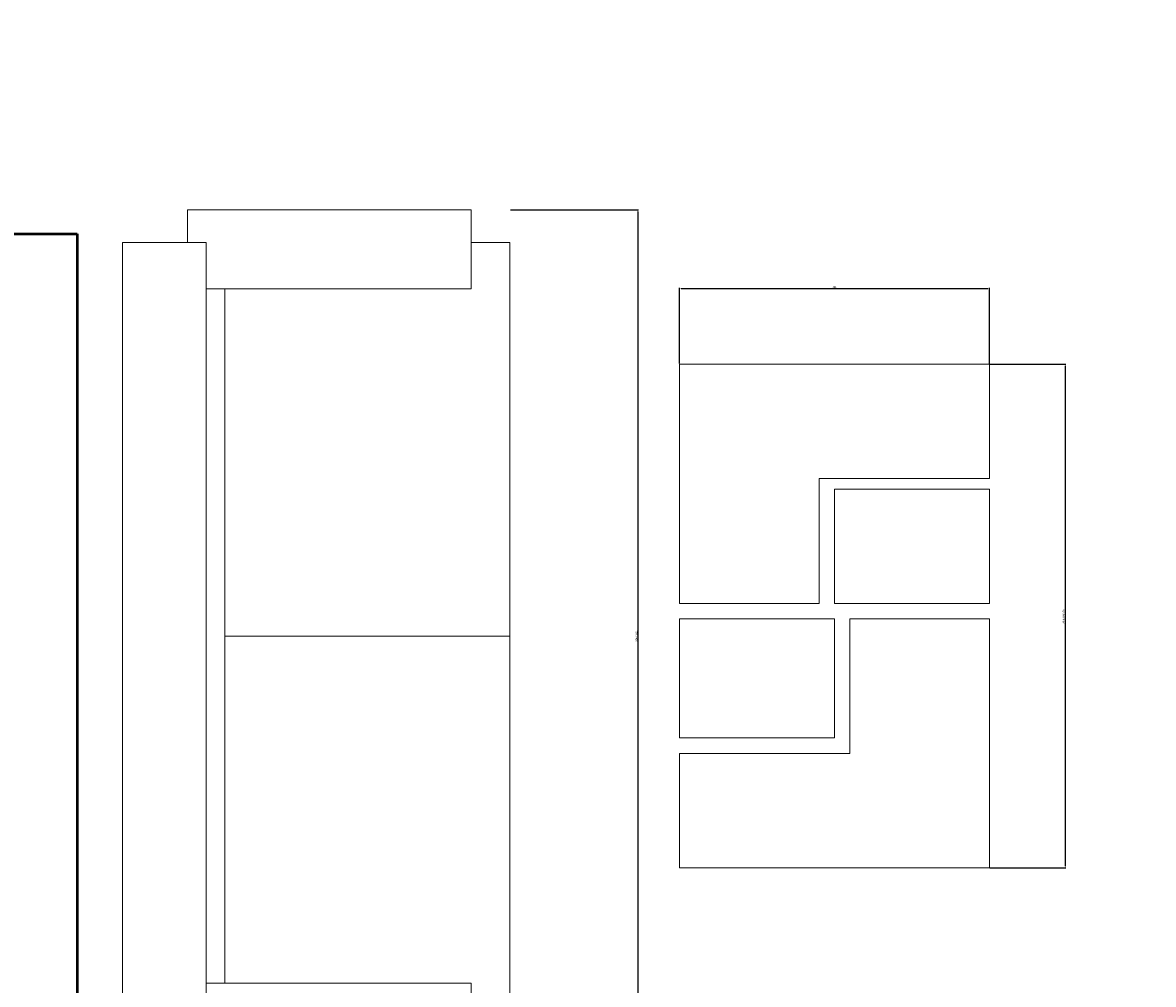
# Model space of a CAD drawing. Units: millimetres. Extents: x -857 to 54106, y -13666 to 13947.
# Tile 9 of 41: x 7333 to 9086, y 6990 to 8482. Entities that reach past the tile are written whole.
import ezdxf

# ---------------------------------------------------------------- set-up
doc = ezdxf.new("R2010")
doc.units = ezdxf.units.MM
for name, color, linetype, lineweight in [('A-ANNO-DIMS', 2, 'Continuous', 18), ('A-FLOR-PATT', 252, 'Continuous', 13), ('A-FURN', 21, 'Continuous', 18), ('A-FURNITURE', 25, 'Continuous', 9), ('A-WALL', 7, 'Continuous', 50)]:
    doc.layers.add(name, color=color, linetype=linetype, lineweight=lineweight)
doc.styles.get("Standard").update_dxf_attribs({"font": 'arial.ttf'})
doc.dimstyles.new('ISO-25', dxfattribs={"dimtxt": 2.5, "dimasz": 2.5, "dimexe": 1.25, "dimexo": 0.625, "dimtad": 1, "dimtxsty": 'Standard', "dimcen": 2.5, "dimadec": 0, "dimazin": 0, "dimtfac": 1, "dimtmove": 0, "dimatfit": 3, "dimfxl": 1, "dimarcsym": 0})

# ---------------------------------------------------------------- blocks, each defined once
blk = doc.blocks.new('A$C0E8E2537')
at = {"layer": 'A-FURNITURE'}
for p, q in [((30.478, 0), (-30.478, 0)), ((-30.478, 0), (-30.478, -6.486)), ((30.478, 0), (30.478, -6.486)), ((-30.478, -5.045), (-33, -5.045)), ((-33, -5.045), (-33, -26.997)), ((30.478, -5.045), (33, -5.045)), ((33, -5.045), (33, -26.997)), ((30.478, -6.486), (-30.478, -6.486)), ((-26.874, -6.486), (-26.874, -7.927)), ((26.874, -6.486), (26.874, -26.997)), ((26.874, -7.927), (-26.874, -7.927)), ((-26.874, -7.927), (-26.874, -26.997)), ((0, -30), (0, -7.927)), ((-33, -26.997), (-26.874, -26.997)), ((-30.478, -26.997), (-30.478, -30)), ((33, -26.997), (26.874, -26.997)), ((30.478, -26.997), (30.478, -30)), ((30.478, -30), (-30.478, -30))]:
    blk.add_line(p, q, dxfattribs=at)
blk = doc.blocks.new('A$C03AA15B9')
at = {"layer": 'A-FURNITURE'}
for points in [[(13.194, 19.718), (13.194, 30.14), (0, 30.14), (0, 38.992), (24, 38.992), (24, 19.718)], [(0, 28.945), (12, 28.945), (12, 19.718), (0, 19.718)], [(10.806, 18.524), (10.806, 8.852), (24, 8.852), (24, 0), (0, 0), (0, 18.524)], [(24, 9.672), (12, 9.672), (12, 18.524), (24, 18.524)]]:
    blk.add_lwpolyline(points, close=True, dxfattribs=at)
blk = doc.blocks.new('*D53')
at = {"layer": 'A-ANNO-DIMS', "color": 0, "lineweight": -2, "transparency": 16777216}
for p, q in [((8089.1, 8191.6), (8288, 8191.6)), ((8286.8, 8189.1), (8286.8, 6871.7)), ((8089.1, 6869.2), (8288, 6869.2))]:
    blk.add_line(p, q, dxfattribs=at)
at = {"layer": 'A-ANNO-DIMS', "color": 0, "transparency": 16777216}
for points in [[(8286.4, 8189.1), (8287.2, 8189.1), (8286.8, 8191.6)], [(8286.4, 6871.7), (8287.2, 6871.7), (8286.8, 6869.2)]]:
    blk.add_solid(points, dxfattribs=at)
at = {"layer": 'Defpoints', "color": 0, "transparency": 16777216}
for p in [(8088.4, 8191.6), (8088.4, 6869.2), (8286.8, 6869.2)]:
    blk.add_point(p, dxfattribs=at)
at = {"layer": 'A-ANNO-DIMS', "color": 0, "transparency": 16777216, "insert": (8284.9, 7530.4), "char_height": 2.5, "attachment_point": 5, "rotation": 90}
blk.add_mtext('SOFA 1322', dxfattribs=at)
blk = doc.blocks.new('*D55')
at = {"layer": 'A-ANNO-DIMS', "color": 0, "lineweight": -2, "transparency": 16777216}
for p, q in [((8832.8, 7952.3), (8950.6, 7952.3)), ((8949.3, 7949.8), (8949.3, 7173.6)), ((8832.8, 7171.1), (8950.6, 7171.1))]:
    blk.add_line(p, q, dxfattribs=at)
at = {"layer": 'A-ANNO-DIMS', "color": 0, "transparency": 16777216}
for points in [[(8948.9, 7949.8), (8949.8, 7949.8), (8949.3, 7952.3)], [(8948.9, 7173.6), (8949.8, 7173.6), (8949.3, 7171.1)]]:
    blk.add_solid(points, dxfattribs=at)
at = {"layer": 'Defpoints', "color": 0, "transparency": 16777216}
for p in [(8832.2, 7952.3), (8832.2, 7171.1), (8949.3, 7171.1)]:
    blk.add_point(p, dxfattribs=at)
at = {"layer": 'A-ANNO-DIMS', "color": 0, "transparency": 16777216, "insert": (8947.4, 7561.7), "char_height": 2.5, "attachment_point": 5, "rotation": 90}
blk.add_mtext('ARMCHAIR 781', dxfattribs=at)
blk = doc.blocks.new('*D56')
at = {"layer": 'A-ANNO-DIMS', "color": 0, "lineweight": -2, "transparency": 16777216}
for p, q in [((8351.3, 7953), (8351.3, 8070.8)), ((8353.8, 8069.5), (8829.7, 8069.5)), ((8832.2, 7953), (8832.2, 8070.8))]:
    blk.add_line(p, q, dxfattribs=at)
at = {"layer": 'A-ANNO-DIMS', "color": 0, "transparency": 16777216}
for points in [[(8353.8, 8069.9), (8353.8, 8069.1), (8351.3, 8069.5)], [(8829.7, 8069.9), (8829.7, 8069.1), (8832.2, 8069.5)]]:
    blk.add_solid(points, dxfattribs=at)
at = {"layer": 'Defpoints', "color": 0, "transparency": 16777216}
for p in [(8832.2, 8069.5), (8351.3, 7952.3), (8832.2, 7952.3)]:
    blk.add_point(p, dxfattribs=at)
at = {"layer": 'A-ANNO-DIMS', "color": 0, "transparency": 16777216, "insert": (8591.7, 8071.4), "char_height": 2.5, "attachment_point": 5}
blk.add_mtext('481', dxfattribs=at)

msp = doc.modelspace()

# ---------------------------------------------------------------- hatches: boundary and pattern name
at = {"layer": 'A-FLOR-PATT'}
h = msp.add_hatch(dxfattribs=at)
h.set_pattern_fill('CROSS', color=256, scale=50)
h.set_pattern_definition([(0, (-5489.92, -2561.3), (317.5, 317.5), [158.75, -476.25]), (90, (-5410.54, -2640.7), (-317.5, 317.5), [158.75, -476.25])])
h.paths.add_polyline_path([(16392.264, 9351.555), (14441.85, 9351.555), (13967.28, 9353.369), (13967.28, 9241.901), (13967.28, 8421.901), (13967.28, 6326.555), (16392.264, 6326.555)])
h.paths.add_polyline_path([(16392.264, 12804.231), (14667.264, 12804.231), (14667.264, 12374.147, -0.32131534), (15142.28, 11711.288), (14667.264, 11711.288), (14667.264, 11601.555), (16392.264, 11601.555)])
h.paths.add_polyline_path([(11417.28, 12804.231), (8617.28, 12804.231), (8617.28, 11804.231), (9371.341, 11804.231), (9371.341, 11750.152), (10571.341, 11750.152), (10571.341, 11804.231), (11417.28, 11804.231)])

# ---------------------------------------------------------------- linework, layer by layer
at = {"layer": 'A-WALL'}
for p, q in [((7192.28, 8154.231), (7417.28, 8154.231)), ((7417.28, 8154.231), (7417.28, 5554.231))]:
    msp.add_line(p, q, dxfattribs=at)

# ---------------------------------------------------------------- block references
at = {"layer": 'A-FURN', "ltscale": 4}
for name, p, xscale, yscale, zscale, rotation in [('A$C0E8E2537', (7487.337, 7530.393), -20.03650789584554, 20.03650789584554, 20.03650789584554, 90), ('A$C03AA15B9', (8351.277, 7952.331), -20.03650789584363, 20.03650789584363, 20.03650789584363, 180)]:
    msp.add_blockref(name, p, dxfattribs=dict(at, xscale=xscale, yscale=yscale, zscale=zscale, rotation=rotation))

# ---------------------------------------------------------------- dimensions: what is measured, and where the dimension line sits
at = {"layer": 'A-ANNO-DIMS'}
for base, p1, p2, text, picture, middle in [((8286.794, 6869.188), (8088.433, 8191.597), (8088.433, 6869.188), 'SOFA <>', '*D53', (8284.875, 7530.393)), ((8949.344, 7171.068), (8832.155, 7952.331), (8832.155, 7171.068), 'ARMCHAIR <>', '*D55', (8947.427, 7561.699))]:
    dim = msp.add_linear_dim(base=base, p1=p1, p2=p2, angle=270, text=text, dimstyle='ISO-25', override={"dimdec": 0, "dimrnd": 0, "dimzin": 0, "dimlunit": 2}, dxfattribs=at)
    dim.commit()
    dim.dimension.update_dxf_attribs({"geometry": picture, "text_midpoint": middle})
dim = msp.add_linear_dim(base=(8832.155, 8069.52), p1=(8351.278, 7952.331), p2=(8832.155, 7952.331), dimstyle='ISO-25', override={"dimdec": 0, "dimrnd": 0, "dimzin": 0, "dimlunit": 2}, dxfattribs=at)
dim.commit()
dim.dimension.update_dxf_attribs({"geometry": '*D56', "text_midpoint": (8591.717, 8071.421)})

doc.saveas('drawing.dxf')
